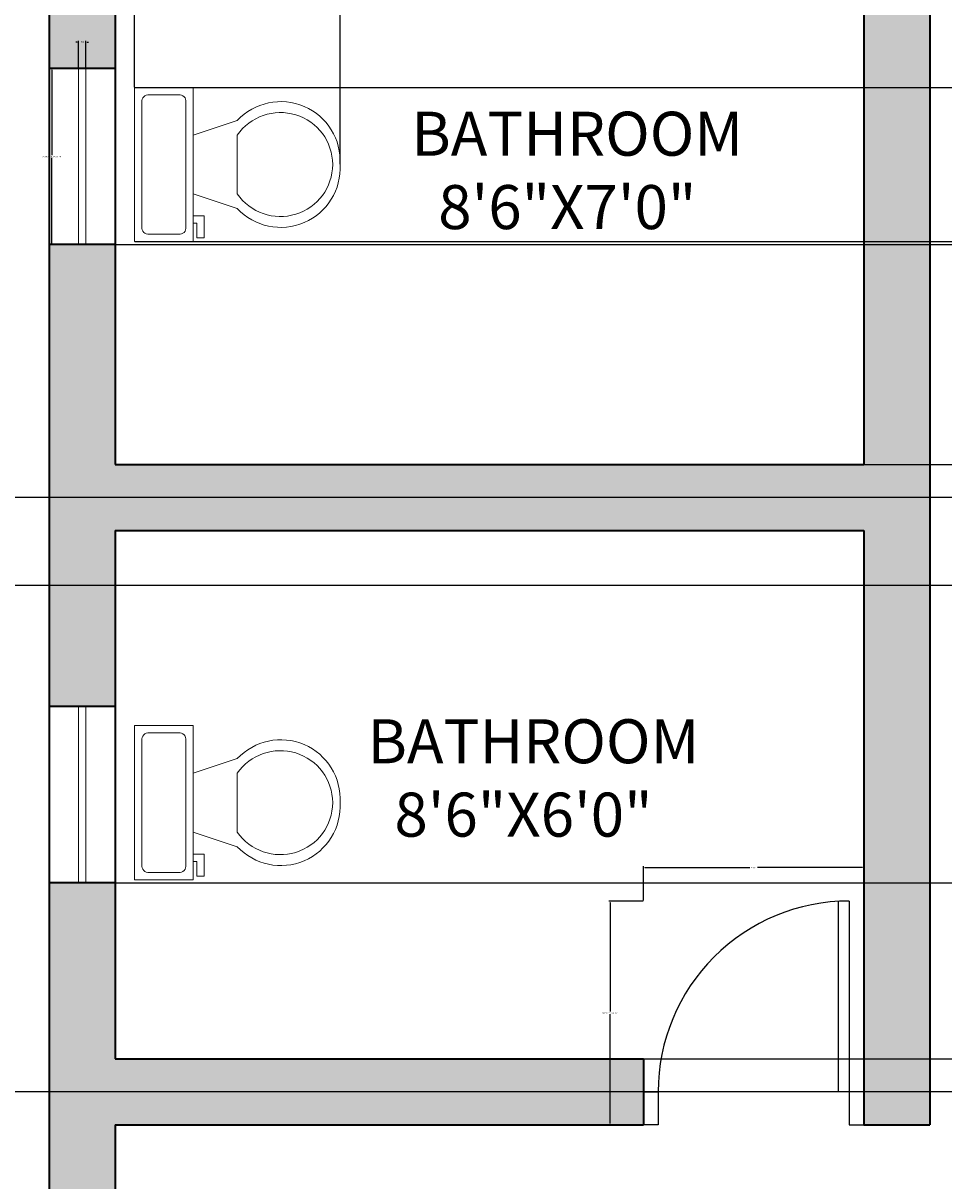
# Model space of a CAD drawing. Units: inches. Extents: x 5716 to 6907, y 12769 to 13594.
# Tile 4 of 17: x 5815 to 5941, y 13109 to 13266. Entities that reach past the tile are written whole.
import ezdxf

# ---------------------------------------------------------------- set-up
doc = ezdxf.new("R2010")
doc.units = ezdxf.units.IN
for name, color, linetype, lineweight in [('A-ANNO-DIMS', 2, 'Continuous', 18), ('A-AREA-IDEN', 7, 'Continuous', 18), ('A-DOOR', 4, 'Continuous', 25), ('A-FLOR-FIXT', 9, 'Continuous', 18), ('A-GLAZ', 4, 'Continuous', 18), ('A-WALL', 7, 'Continuous', 35), ('A-WALL-PATT', 252, 'Continuous', 13)]:
    doc.layers.add(name, color=color, linetype=linetype, lineweight=lineweight)
doc.styles.get("Standard").update_dxf_attribs({"font": 'arial.ttf'})
doc.dimstyles.get("Standard").update_dxf_attribs({"dimtxt": 0.18, "dimasz": 0.18, "dimexe": 0.18, "dimexo": 0.0625, "dimgap": 0.09, "dimtad": 0, "dimtih": 1, "dimtoh": 1, "dimdec": 4, "dimzin": 0, "dimdsep": 46, "dimtxsty": 'Standard', "dimcen": 0.09, "dimadec": 0, "dimazin": 0, "dimtfac": 1, "dimtdec": 4, "dimtofl": 0, "dimtmove": 0, "dimatfit": 3, "dimfxl": 1, "dimtolj": 1, "dimtzin": 0, "dimarcsym": 0})

# ---------------------------------------------------------------- blocks, each defined once
blk = doc.blocks.new('*U11')
for p, q in [((9.5, -6), (9.5, -2)), ((-10, -8.5), (-8, -8.5)), ((-10, -9.5), (-10, -8.5)), ((-8, -8.5), (-8, -8)), ((-7, -8), (-7, -9.5)), ((-4, -8), (-6, -14)), ((4, -8), (6, -14)), ((-7, -9.5), (-10, -9.5)), ((4, -14), (-4, -14))]:
    blk.add_line(p, q)
blk.add_lwpolyline([(10.5, -8), (10.5, 0), (-10.5, 0), (-10.5, -8)], close=True)
for points in [[(8.5, -1), (-8.5, -1)], [(-9.5, -2), (-9.5, -6)], [(-8.5, -7), (8.5, -7)]]:
    blk.add_lwpolyline(points)
for centre, radius, start, end in [((-8.625, -1.875), 0.8839, 81.8699, 188.1301), ((8.625, -1.875), 0.8839, 351.8699, 98.1301), ((-8.625, -6.125), 0.8839, 171.869898, 278.1301), ((8.625, -6.125), 0.8839, 261.8699, 8.1301), ((-0.4772, -19.9188), 8.0953, 133.01722, 273.38), ((0.0374, -19.8731), 7.127, 124.50543, 269.7), ((-0.0373, -19.8731), 7.127, 270.3, 55.4946), ((0.4773, -19.9188), 8.0953, 266.62, 46.9828)]:
    blk.add_arc(centre, radius, start, end)
blk = doc.blocks.new('DOOR-SWING-30IN')
for p, q in [((0, 4.5), (-2, 4.5)), ((0, 0), (0, 4.5)), ((26, 0), (26, 4.5)), ((26, 4.5), (28, 4.5)), ((-2, 0), (0, 0)), ((0, -26), (0, 0)), ((0, 0), (1.5, 0)), ((1.5, -25.96), (1.5, 0)), ((28, 0), (26, 0))]:
    blk.add_line(p, q)
blk.add_arc((0, 0), 26, 270, 0)
blk = doc.blocks.new('WIN-GLAZING-24IN')
for p, q in [((0, 0), (0, -24)), ((1, 0), (1, -24))]:
    blk.add_line(p, q)
blk = doc.blocks.new('*D21')
at = {"layer": 'A-ANNO-DIMS', "color": 0, "lineweight": -2, "transparency": 16777216}
for p, q in [((5899.96, 13146.65), (5895.27, 13146.65)), ((5895.45, 13146.47), (5895.45, 13131.58)), ((5895.45, 13116.33), (5895.45, 13131.22)), ((5899.96, 13116.15), (5895.27, 13116.15))]:
    blk.add_line(p, q, dxfattribs=at)
at = {"layer": 'A-ANNO-DIMS', "color": 0, "transparency": 16777216}
for points in [[(5895.42, 13146.47), (5895.48, 13146.47), (5895.45, 13146.65)], [(5895.42, 13116.33), (5895.48, 13116.33), (5895.45, 13116.15)]]:
    blk.add_solid(points, dxfattribs=at)
at = {"layer": 'Defpoints', "color": 0, "transparency": 16777216}
for p in [(5900.02, 13146.65), (5895.45, 13116.15), (5900.02, 13116.15)]:
    blk.add_point(p, dxfattribs=at)
at = {"layer": 'A-ANNO-DIMS', "color": 0, "transparency": 16777216, "insert": (5895.45, 13131.4), "char_height": 0.18, "attachment_point": 5}
blk.add_mtext('\\A1;BATH DOOR 31 TYP.', dxfattribs=at)
blk = doc.blocks.new('*D22')
at = {"layer": 'A-ANNO-DIMS', "color": 0, "lineweight": -2, "transparency": 16777216}
for p, q in [((5900.02, 13146.71), (5900.02, 13151.4)), ((5900.2, 13151.22), (5914.49, 13151.22)), ((5929.84, 13151.22), (5915.55, 13151.22)), ((5930.02, 13146.71), (5930.02, 13151.4))]:
    blk.add_line(p, q, dxfattribs=at)
at = {"layer": 'A-ANNO-DIMS', "color": 0, "transparency": 16777216}
for points in [[(5900.2, 13151.25), (5900.2, 13151.19), (5900.02, 13151.22)], [(5929.84, 13151.25), (5929.84, 13151.19), (5930.02, 13151.22)]]:
    blk.add_solid(points, dxfattribs=at)
at = {"layer": 'Defpoints', "color": 0, "transparency": 16777216}
for p in [(5900.02, 13151.22), (5900.02, 13146.65), (5930.02, 13146.65)]:
    blk.add_point(p, dxfattribs=at)
at = {"layer": 'A-ANNO-DIMS', "color": 0, "transparency": 16777216, "insert": (5915.02, 13151.22), "char_height": 0.18, "attachment_point": 5}
blk.add_mtext('\\A1;30 TYP.', dxfattribs=at)
blk = doc.blocks.new('*D29')
at = {"layer": 'A-ANNO-DIMS', "color": 0, "lineweight": -2, "transparency": 16777216}
for p, q in [((5822.96, 13260.15), (5819.24, 13260.15)), ((5819.42, 13259.97), (5819.42, 13248.33)), ((5819.42, 13236.33), (5819.42, 13247.97)), ((5822.96, 13236.15), (5819.24, 13236.15))]:
    blk.add_line(p, q, dxfattribs=at)
at = {"layer": 'A-ANNO-DIMS', "color": 0, "transparency": 16777216}
for points in [[(5819.39, 13259.97), (5819.45, 13259.97), (5819.42, 13260.15)], [(5819.39, 13236.33), (5819.45, 13236.33), (5819.42, 13236.15)]]:
    blk.add_solid(points, dxfattribs=at)
at = {"layer": 'Defpoints', "color": 0, "transparency": 16777216}
for p in [(5823.02, 13260.15), (5819.42, 13236.15), (5823.02, 13236.15)]:
    blk.add_point(p, dxfattribs=at)
at = {"layer": 'A-ANNO-DIMS', "color": 0, "transparency": 16777216, "insert": (5819.42, 13248.15), "char_height": 0.18, "attachment_point": 5}
blk.add_mtext('\\A1;BATH WINDOW 24 TYP.', dxfattribs=at)
blk = doc.blocks.new('*D30')
at = {"layer": 'A-ANNO-DIMS', "color": 0, "lineweight": -2, "transparency": 16777216}
for p, q in [((5822.84, 13263.75), (5822.66, 13263.75)), ((5823.02, 13260.21), (5823.02, 13263.93)), ((5824.02, 13260.21), (5824.02, 13263.93)), ((5824.2, 13263.75), (5824.38, 13263.75))]:
    blk.add_line(p, q, dxfattribs=at)
at = {"layer": 'A-ANNO-DIMS', "color": 0, "transparency": 16777216}
for points in [[(5822.84, 13263.78), (5822.84, 13263.72), (5823.02, 13263.75)], [(5824.2, 13263.78), (5824.2, 13263.72), (5824.02, 13263.75)]]:
    blk.add_solid(points, dxfattribs=at)
at = {"layer": 'Defpoints', "color": 0, "transparency": 16777216}
for p in [(5823.02, 13263.75), (5823.02, 13260.15), (5824.02, 13260.15)]:
    blk.add_point(p, dxfattribs=at)
at = {"layer": 'A-ANNO-DIMS', "color": 0, "transparency": 16777216, "insert": (5823.52, 13263.75), "char_height": 0.18, "attachment_point": 5}
blk.add_mtext('\\A1;1 TYP.', dxfattribs=at)
blk = doc.blocks.new('*D50')
at = {"layer": 'A-ANNO-DIMS', "color": 0, "lineweight": -2, "transparency": 16777216}
for p, q in [((5818.96, 13440.15), (5716.04, 13440.15)), ((5716.22, 13439.97), (5716.22, 13140.83)), ((5716.22, 12841.33), (5716.22, 13140.47)), ((5818.96, 12841.15), (5716.04, 12841.15))]:
    blk.add_line(p, q, dxfattribs=at)
at = {"layer": 'A-ANNO-DIMS', "color": 0, "transparency": 16777216}
for points in [[(5716.19, 13439.97), (5716.25, 13439.97), (5716.22, 13440.15)], [(5716.19, 12841.33), (5716.25, 12841.33), (5716.22, 12841.15)]]:
    blk.add_solid(points, dxfattribs=at)
at = {"layer": 'Defpoints', "color": 0, "transparency": 16777216}
for p in [(5716.22, 13440.15), (5819.02, 13440.15), (5819.02, 12841.15)]:
    blk.add_point(p, dxfattribs=at)
at = {"layer": 'A-ANNO-DIMS', "color": 0, "transparency": 16777216, "insert": (5716.22, 13140.65), "char_height": 0.18, "attachment_point": 5}
blk.add_mtext('\\A1;599', dxfattribs=at)
blk = doc.blocks.new('*D51')
at = {"layer": 'A-ANNO-DIMS', "color": 0, "lineweight": -2, "transparency": 16777216}
for p, q in [((5819.02, 13440.21), (5819.02, 13594.38)), ((5819.2, 13594.2), (6033.23, 13594.2)), ((6247.84, 13594.2), (6033.82, 13594.2)), ((6248.02, 13194.21), (6248.02, 13594.38))]:
    blk.add_line(p, q, dxfattribs=at)
at = {"layer": 'A-ANNO-DIMS', "color": 0, "transparency": 16777216}
for points in [[(5819.2, 13594.23), (5819.2, 13594.17), (5819.02, 13594.2)], [(6247.84, 13594.23), (6247.84, 13594.17), (6248.02, 13594.2)]]:
    blk.add_solid(points, dxfattribs=at)
at = {"layer": 'Defpoints', "color": 0, "transparency": 16777216}
for p in [(6248.02, 13594.2), (5819.02, 13440.15), (6248.02, 13194.15)]:
    blk.add_point(p, dxfattribs=at)
at = {"layer": 'A-ANNO-DIMS', "color": 0, "transparency": 16777216, "insert": (6033.52, 13594.2), "char_height": 0.18, "attachment_point": 5}
blk.add_mtext('\\A1;429', dxfattribs=at)
blk = doc.blocks.new('*D52')
at = {"layer": 'A-ANNO-DIMS', "color": 0, "lineweight": -2, "transparency": 16777216}
for p, q in [((6267.34, 13440.15), (5716.04, 13440.15)), ((5716.22, 13439.97), (5716.22, 13140.83)), ((5716.22, 12841.33), (5716.22, 13140.47)), ((6267.34, 12841.15), (5716.04, 12841.15))]:
    blk.add_line(p, q, dxfattribs=at)
at = {"layer": 'A-ANNO-DIMS', "color": 0, "transparency": 16777216}
for points in [[(5716.19, 13439.97), (5716.25, 13439.97), (5716.22, 13440.15)], [(5716.19, 12841.33), (5716.25, 12841.33), (5716.22, 12841.15)]]:
    blk.add_solid(points, dxfattribs=at)
at = {"layer": 'Defpoints', "color": 0, "transparency": 16777216}
for p in [(6267.41, 13440.15), (5716.22, 12841.15), (6267.41, 12841.15)]:
    blk.add_point(p, dxfattribs=at)
at = {"layer": 'A-ANNO-DIMS', "color": 0, "transparency": 16777216, "insert": (5716.22, 13140.65), "char_height": 0.18, "attachment_point": 5}
blk.add_mtext('\\A1;599', dxfattribs=at)
blk = doc.blocks.new('*D59')
at = {"layer": 'A-ANNO-DIMS', "color": 0, "lineweight": -2, "transparency": 16777216}
for p, q in [((6736.67, 13294.65), (5716.04, 13294.65)), ((5716.22, 13294.47), (5716.22, 13248.33)), ((5716.22, 13201.83), (5716.22, 13247.97)), ((6736.67, 13201.65), (5716.04, 13201.65))]:
    blk.add_line(p, q, dxfattribs=at)
at = {"layer": 'A-ANNO-DIMS', "color": 0, "transparency": 16777216}
for points in [[(5716.19, 13294.47), (5716.25, 13294.47), (5716.22, 13294.65)], [(5716.19, 13201.83), (5716.25, 13201.83), (5716.22, 13201.65)]]:
    blk.add_solid(points, dxfattribs=at)
at = {"layer": 'Defpoints', "color": 0, "transparency": 16777216}
for p in [(6736.73, 13294.65), (5716.22, 13201.65), (6736.73, 13201.65)]:
    blk.add_point(p, dxfattribs=at)
at = {"layer": 'A-ANNO-DIMS', "color": 0, "transparency": 16777216, "insert": (5716.22, 13248.15), "char_height": 0.18, "attachment_point": 5}
blk.add_mtext('\\A1;93', dxfattribs=at)
blk = doc.blocks.new('*D60')
at = {"layer": 'A-ANNO-DIMS', "color": 0, "lineweight": -2, "transparency": 16777216}
for p, q in [((6736.67, 13201.65), (5716.04, 13201.65)), ((5716.22, 13201.47), (5716.22, 13195.83)), ((5716.22, 13189.83), (5716.22, 13195.47)), ((6827.78, 13189.65), (5716.04, 13189.65))]:
    blk.add_line(p, q, dxfattribs=at)
at = {"layer": 'A-ANNO-DIMS', "color": 0, "transparency": 16777216}
for points in [[(5716.19, 13201.47), (5716.25, 13201.47), (5716.22, 13201.65)], [(5716.19, 13189.83), (5716.25, 13189.83), (5716.22, 13189.65)]]:
    blk.add_solid(points, dxfattribs=at)
at = {"layer": 'Defpoints', "color": 0, "transparency": 16777216}
for p in [(6736.73, 13201.65), (5716.22, 13189.65), (6827.84, 13189.65)]:
    blk.add_point(p, dxfattribs=at)
at = {"layer": 'A-ANNO-DIMS', "color": 0, "transparency": 16777216, "insert": (5716.22, 13195.65), "char_height": 0.18, "attachment_point": 5}
blk.add_mtext('\\A1;12', dxfattribs=at)
blk = doc.blocks.new('*D61')
at = {"layer": 'A-ANNO-DIMS', "color": 0, "lineweight": -2, "transparency": 16777216}
for p, q in [((6827.78, 13189.65), (5716.04, 13189.65)), ((5716.22, 13189.47), (5716.22, 13155.33)), ((5716.22, 13120.83), (5716.22, 13154.97)), ((6736.67, 13120.65), (5716.04, 13120.65))]:
    blk.add_line(p, q, dxfattribs=at)
at = {"layer": 'A-ANNO-DIMS', "color": 0, "transparency": 16777216}
for points in [[(5716.19, 13189.47), (5716.25, 13189.47), (5716.22, 13189.65)], [(5716.19, 13120.83), (5716.25, 13120.83), (5716.22, 13120.65)]]:
    blk.add_solid(points, dxfattribs=at)
at = {"layer": 'Defpoints', "color": 0, "transparency": 16777216}
for p in [(6827.84, 13189.65), (5716.22, 13120.65), (6736.73, 13120.65)]:
    blk.add_point(p, dxfattribs=at)
at = {"layer": 'A-ANNO-DIMS', "color": 0, "transparency": 16777216, "insert": (5716.22, 13155.15), "char_height": 0.18, "attachment_point": 5}
blk.add_mtext('\\A1;69', dxfattribs=at)
blk = doc.blocks.new('*D62')
at = {"layer": 'A-ANNO-DIMS', "color": 0, "lineweight": -2, "transparency": 16777216}
for p, q in [((6736.67, 13120.65), (5716.04, 13120.65)), ((5716.22, 13120.47), (5716.22, 13100.33)), ((5716.22, 13079.83), (5716.22, 13099.97)), ((6736.67, 13079.65), (5716.04, 13079.65))]:
    blk.add_line(p, q, dxfattribs=at)
at = {"layer": 'A-ANNO-DIMS', "color": 0, "transparency": 16777216}
for points in [[(5716.19, 13120.47), (5716.25, 13120.47), (5716.22, 13120.65)], [(5716.19, 13079.83), (5716.25, 13079.83), (5716.22, 13079.65)]]:
    blk.add_solid(points, dxfattribs=at)
at = {"layer": 'Defpoints', "color": 0, "transparency": 16777216}
for p in [(6736.73, 13120.65), (5716.22, 13079.65), (6736.73, 13079.65)]:
    blk.add_point(p, dxfattribs=at)
at = {"layer": 'A-ANNO-DIMS', "color": 0, "transparency": 16777216, "insert": (5716.22, 13100.15), "char_height": 0.18, "attachment_point": 5}
blk.add_mtext('\\A1;41', dxfattribs=at)
blk = doc.blocks.new('*D69')
at = {"layer": 'A-ANNO-DIMS', "color": 0, "lineweight": -2, "transparency": 16777216}
for p, q in [((5828.09, 13149.15), (6907.26, 13149.15)), ((6907.08, 13148.97), (6907.08, 13137.33)), ((6907.08, 13125.33), (6907.08, 13136.97)), ((5828.09, 13125.15), (6907.26, 13125.15))]:
    blk.add_line(p, q, dxfattribs=at)
at = {"layer": 'A-ANNO-DIMS', "color": 0, "transparency": 16777216}
for points in [[(6907.05, 13148.97), (6907.11, 13148.97), (6907.08, 13149.15)], [(6907.05, 13125.33), (6907.11, 13125.33), (6907.08, 13125.15)]]:
    blk.add_solid(points, dxfattribs=at)
at = {"layer": 'Defpoints', "color": 0, "transparency": 16777216}
for p in [(5828.02, 13149.15), (6907.08, 13149.15), (5828.02, 13125.15)]:
    blk.add_point(p, dxfattribs=at)
at = {"layer": 'A-ANNO-DIMS', "color": 0, "transparency": 16777216, "insert": (6907.08, 13137.15), "char_height": 0.18, "attachment_point": 5}
blk.add_mtext('\\A1;24', dxfattribs=at)
blk = doc.blocks.new('*D70')
at = {"layer": 'A-ANNO-DIMS', "color": 0, "lineweight": -2, "transparency": 16777216}
for p, q in [((5828.09, 13236.15), (6907.26, 13236.15)), ((6907.08, 13235.97), (6907.08, 13221.33)), ((6907.08, 13206.33), (6907.08, 13220.97)), ((5828.09, 13206.15), (6907.26, 13206.15))]:
    blk.add_line(p, q, dxfattribs=at)
at = {"layer": 'A-ANNO-DIMS', "color": 0, "transparency": 16777216}
for points in [[(6907.05, 13235.97), (6907.11, 13235.97), (6907.08, 13236.15)], [(6907.05, 13206.33), (6907.11, 13206.33), (6907.08, 13206.15)]]:
    blk.add_solid(points, dxfattribs=at)
at = {"layer": 'Defpoints', "color": 0, "transparency": 16777216}
for p in [(5828.02, 13236.15), (6907.08, 13236.15), (5828.02, 13206.15)]:
    blk.add_point(p, dxfattribs=at)
at = {"layer": 'A-ANNO-DIMS', "color": 0, "transparency": 16777216, "insert": (6907.08, 13221.15), "char_height": 0.18, "attachment_point": 5}
blk.add_mtext('\\A1;30', dxfattribs=at)
blk = doc.blocks.new('*D75')
at = {"layer": 'A-ANNO-DIMS', "color": 0, "lineweight": -2, "transparency": 16777216}
for p, q in [((5830.67, 13257.62), (5830.67, 13594.38)), ((5830.85, 13594.2), (5844.45, 13594.2)), ((5858.49, 13594.2), (5844.89, 13594.2)), ((5858.67, 13247.12), (5858.67, 13594.38))]:
    blk.add_line(p, q, dxfattribs=at)
at = {"layer": 'A-ANNO-DIMS', "color": 0, "transparency": 16777216}
for points in [[(5830.85, 13594.23), (5830.85, 13594.17), (5830.67, 13594.2)], [(5858.49, 13594.23), (5858.49, 13594.17), (5858.67, 13594.2)]]:
    blk.add_solid(points, dxfattribs=at)
at = {"layer": 'Defpoints', "color": 0, "transparency": 16777216}
for p in [(5858.67, 13594.2), (5830.67, 13257.56), (5858.67, 13247.06)]:
    blk.add_point(p, dxfattribs=at)
at = {"layer": 'A-ANNO-DIMS', "color": 0, "transparency": 16777216, "insert": (5844.67, 13594.2), "char_height": 0.18, "attachment_point": 5}
blk.add_mtext('\\A1;28', dxfattribs=at)
blk = doc.blocks.new('*D76')
at = {"layer": 'A-ANNO-DIMS', "color": 0, "lineweight": -2, "transparency": 16777216}
for p, q in [((5830.73, 13257.56), (6907.26, 13257.56)), ((6907.08, 13257.38), (6907.08, 13247.24)), ((6907.08, 13236.74), (6907.08, 13246.88)), ((5830.73, 13236.56), (6907.26, 13236.56))]:
    blk.add_line(p, q, dxfattribs=at)
at = {"layer": 'A-ANNO-DIMS', "color": 0, "transparency": 16777216}
for points in [[(6907.05, 13257.38), (6907.11, 13257.38), (6907.08, 13257.56)], [(6907.05, 13236.74), (6907.11, 13236.74), (6907.08, 13236.56)]]:
    blk.add_solid(points, dxfattribs=at)
at = {"layer": 'Defpoints', "color": 0, "transparency": 16777216}
for p in [(5830.67, 13257.56), (5830.67, 13236.56), (6907.08, 13236.56)]:
    blk.add_point(p, dxfattribs=at)
at = {"layer": 'A-ANNO-DIMS', "color": 0, "transparency": 16777216, "insert": (6907.08, 13247.06), "char_height": 0.18, "attachment_point": 5}
blk.add_mtext('\\A1;21', dxfattribs=at)

msp = doc.modelspace()

# ---------------------------------------------------------------- hatches: boundary and pattern name
at = {"layer": 'A-WALL-PATT'}
h = msp.add_hatch(color=256, dxfattribs=at)
h.dxf.hatch_style = 1
h.paths.add_polyline_path([(5828.02, 13359.15), (5819.02, 13359.15), (5819.02, 13260.15), (5828.02, 13260.15), (5828.02, 13290.15), (5900.02, 13290.15), (5900.02, 13299.15), (5828.02, 13299.15)])
h = msp.add_hatch(color=256, dxfattribs=at)
h.dxf.hatch_style = 1
h.paths.add_polyline_path([(5939.02, 13290.15), (5966.02, 13290.15), (5966.02, 13299.15), (5930.02, 13299.15), (5930.02, 13206.15), (5828.02, 13206.15), (5828.02, 13236.15), (5819.02, 13236.15), (5819.02, 13173.15), (5828.02, 13173.15), (5828.02, 13197.15), (5930.02, 13197.15), (5930.02, 13116.15), (5939.02, 13116.15)])
h = msp.add_hatch(color=256, dxfattribs=at)
h.dxf.hatch_style = 1
h.paths.add_polyline_path([(5900.02, 13125.15), (5828.02, 13125.15), (5828.02, 13149.15), (5819.02, 13149.15), (5819.02, 13065.65), (5828.02, 13065.65), (5828.02, 13116.15), (5900.02, 13116.15)])

# ---------------------------------------------------------------- linework, layer by layer
at = {"layer": 'A-WALL'}
for p, q in [((5819.02, 13440.15), (5819.02, 12841.15)), ((5930.02, 13299.15), (5930.02, 13206.15)), ((5828.02, 13290.15), (5828.02, 13206.15)), ((5939.02, 13290.15), (5939.02, 13116.15)), ((5828.02, 13260.15), (5819.02, 13260.15)), ((5828.02, 13236.15), (5819.02, 13236.15)), ((5828.02, 13206.15), (5930.02, 13206.15)), ((5828.02, 13197.15), (5930.02, 13197.15)), ((5828.02, 13197.15), (5828.02, 13125.15)), ((5930.02, 13197.15), (5930.02, 13116.15)), ((5828.02, 13173.15), (5819.02, 13173.15)), ((5828.02, 13149.15), (5819.02, 13149.15)), ((5828.02, 13125.15), (5900.02, 13125.15)), ((5900.02, 13125.15), (5900.02, 13116.15)), ((5828.02, 13116.15), (5900.02, 13116.15)), ((5828.02, 13116.15), (5828.02, 12943.15)), ((5930.02, 13116.15), (5939.02, 13116.15))]:
    msp.add_line(p, q, dxfattribs=at)

# ---------------------------------------------------------------- block references
at = {"layer": 'A-DOOR', "rotation": 180}
msp.add_blockref('DOOR-SWING-30IN', (5928.02, 13120.65), dxfattribs=at)
at = {"layer": 'A-FLOR-FIXT', "rotation": 90}
for p in [(5830.67, 13247.06), (5830.67, 13160.06)]:
    msp.add_blockref('*U11', p, dxfattribs=at)
at = {"layer": 'A-GLAZ', "rotation": 180}
msp.add_blockref('WIN-GLAZING-24IN', (5824.02, 13236.15), dxfattribs=at)
at = {"layer": 'A-GLAZ'}
msp.add_blockref('WIN-GLAZING-24IN', (5823.02, 13173.15), dxfattribs=at)

# ---------------------------------------------------------------- texts
at = {"layer": 'A-AREA-IDEN', "char_height": 6, "attachment_point": 1}
for s, width, insert in [('BATHROOM\\P  8\'6"X7\'0"', 76.3009, (5868.38, 13254.26)), ('BATHROOM\\P  8\'6"X6\'0"', 67.4254, (5862.41, 13171.43))]:
    msp.add_mtext_dynamic_manual_height_columns(s, width=width, gutter_width=12.5, heights=[0], dxfattribs=dict(at, insert=insert))

# ---------------------------------------------------------------- dimensions: what is measured, and where the dimension line sits
at = {"layer": 'A-ANNO-DIMS'}
for base, p1, p2, picture, middle in [((6248.02, 13594.2), (5819.02, 13440.15), (6248.02, 13194.15), '*D51', (6033.52, 13594.2)), ((5858.67, 13594.2), (5830.67, 13257.56), (5858.67, 13247.06), '*D75', (5844.67, 13594.2))]:
    dim = msp.add_linear_dim(base=base, p1=p1, p2=p2, dimstyle='Standard', override={"dimdec": 0, "dimlfac": 1, "dimrnd": 0, "dimzin": 0, "dimdsep": 46, "dimlunit": 2}, dxfattribs=at)
    dim.commit()
    dim.dimension.update_dxf_attribs({"geometry": picture, "text_midpoint": middle})
for base, p1, p2, picture, middle in [((5716.22, 13440.15), (5819.02, 12841.15), (5819.02, 13440.15), '*D50', (5716.22, 13140.65)), ((5716.22, 12841.15), (6267.41, 13440.15), (6267.41, 12841.15), '*D52', (5716.22, 13140.65)), ((5716.22, 13201.65), (6736.73, 13294.65), (6736.73, 13201.65), '*D59', (5716.22, 13248.15)), ((6907.08, 13236.56), (5830.67, 13257.56), (5830.67, 13236.56), '*D76', (6907.08, 13247.06)), ((6907.08, 13236.15), (5828.02, 13206.15), (5828.02, 13236.15), '*D70', (6907.08, 13221.15)), ((5716.22, 13189.65), (6736.73, 13201.65), (6827.84, 13189.65), '*D60', (5716.22, 13195.65)), ((5716.22, 13120.65), (6827.84, 13189.65), (6736.73, 13120.65), '*D61', (5716.22, 13155.15)), ((6907.08, 13149.15), (5828.02, 13125.15), (5828.02, 13149.15), '*D69', (6907.08, 13137.15)), ((5716.22, 13079.65), (6736.73, 13120.65), (6736.73, 13079.65), '*D62', (5716.22, 13100.15))]:
    dim = msp.add_linear_dim(base=base, p1=p1, p2=p2, angle=90, dimstyle='Standard', override={"dimdec": 0, "dimlfac": 1, "dimrnd": 0, "dimzin": 0, "dimdsep": 46, "dimlunit": 2}, dxfattribs=at)
    dim.commit()
    dim.dimension.update_dxf_attribs({"geometry": picture, "text_midpoint": middle})
for base, p1, p2, angle, text, picture, middle in [((5823.02, 13263.75), (5824.02, 13260.15), (5823.02, 13260.15), 180, '<> TYP.', '*D30', (5823.52, 13263.75)), ((5819.42, 13236.15), (5823.02, 13260.15), (5823.02, 13236.15), 270, 'BATH WINDOW <> TYP.', '*D29', (5819.42, 13248.15)), ((5900.02, 13151.22), (5930.02, 13146.65), (5900.02, 13146.65), 180, '<> TYP.', '*D22', (5915.02, 13151.22)), ((5895.44751723, 13116.14894948), (5900.02251723, 13146.64894948), (5900.02251723, 13116.14894948), 270, 'BATH DOOR <> TYP.', '*D21', (5895.44751723, 13131.39894948))]:
    dim = msp.add_linear_dim(base=base, p1=p1, p2=p2, angle=angle, text=text, dimstyle='Standard', override={"dimdec": 0, "dimlfac": 1, "dimrnd": 0, "dimzin": 0, "dimdsep": 46, "dimlunit": 2}, dxfattribs=at)
    dim.commit()
    dim.dimension.update_dxf_attribs({"geometry": picture, "text_midpoint": middle})

doc.saveas('drawing.dxf')
